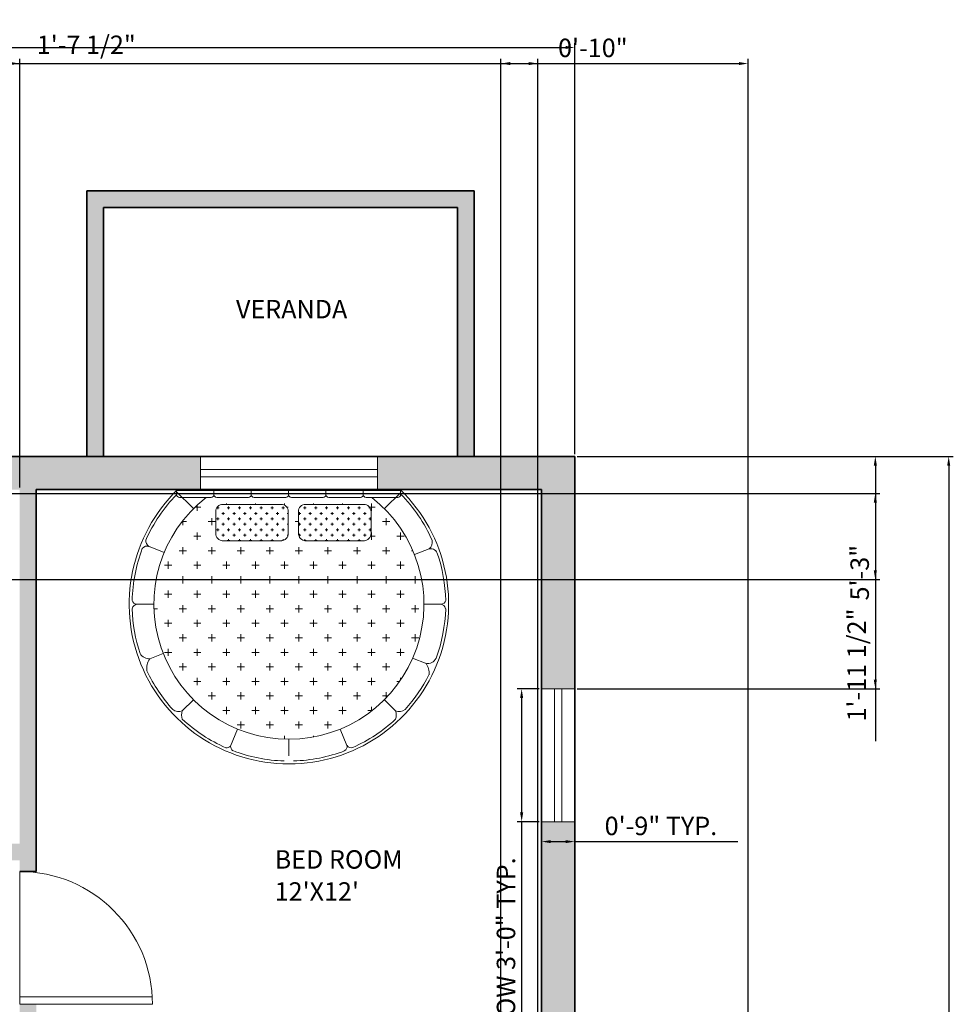
# Model space of a CAD drawing. Units: inches. Extents: x 2923 to 3500, y 1684 to 2381.
# Tile 12 of 12: x 3247 to 3500, y 2114 to 2381. Entities that reach past the tile are written whole.
import ezdxf

# ---------------------------------------------------------------- set-up
doc = ezdxf.new("R2010")
doc.units = ezdxf.units.IN
for name, color, linetype, lineweight in [('A-ANNO-DIMS', 2, 'Continuous', 18), ('A-AREA-IDEN', 7, 'Continuous', 18), ('A-DOOR', 3, 'Continuous', 18), ('A-FURN-PATT', 8, 'Continuous', 13), ('A-GLAZ', 4, 'Continuous', 18), ('A-WALL', 7, 'Continuous', 35), ('A-WALL-PATT', 9, 'Continuous', 13), ('Furniture', 7, 'Continuous', 15)]:
    doc.layers.add(name, color=color, linetype=linetype, lineweight=lineweight)
doc.styles.get("Standard").update_dxf_attribs({"font": 'txt', "height": 5})
doc.dimstyles.new('ISO-25', dxfattribs={"dimtxt": 5, "dimasz": 2.5, "dimexe": 1.25, "dimexo": 0.625, "dimtad": 1, "dimlunit": 3, "dimtxsty": 'Standard', "dimcen": 2.5, "dimadec": 0, "dimazin": 0, "dimtfac": 1, "dimtmove": 0, "dimatfit": 3, "dimfxl": 1, "dimarcsym": 0})

# ---------------------------------------------------------------- blocks, each defined once
blk = doc.blocks.new('*D2')
at = {"layer": 'A-ANNO-DIMS', "color": 0, "lineweight": -2, "transparency": 16777216}
for p, q in [((2969.23, 2263.03), (2969.23, 2374.52)), ((2971.73, 2373.27), (3394.73, 2373.27)), ((3397.23, 2263.03), (3397.23, 2374.52))]:
    blk.add_line(p, q, dxfattribs=at)
at = {"layer": 'A-ANNO-DIMS', "color": 0, "transparency": 16777216}
for points in [[(2971.73, 2373.69), (2971.73, 2372.86), (2969.23, 2373.27)], [(3394.73, 2373.69), (3394.73, 2372.86), (3397.23, 2373.27)]]:
    blk.add_solid(points, dxfattribs=at)
at = {"layer": 'Defpoints', "color": 0, "transparency": 16777216}
for p in [(3397.23, 2373.27), (2969.23, 2262.41), (3397.23, 2262.41)]:
    blk.add_point(p, dxfattribs=at)
at = {"layer": 'A-ANNO-DIMS', "color": 0, "transparency": 16777216, "insert": (3183.23, 2376.87), "char_height": 5, "attachment_point": 5}
blk.add_mtext('35\'-8"', dxfattribs=at)
blk = doc.blocks.new('*D3')
at = {"layer": 'A-ANNO-DIMS', "color": 0, "lineweight": -2, "transparency": 16777216}
for p, q in [((3397.85, 2262.41), (3499.87, 2262.41)), ((3498.62, 2259.91), (3498.62, 1819.91)), ((3397.85, 1817.41), (3499.87, 1817.41))]:
    blk.add_line(p, q, dxfattribs=at)
at = {"layer": 'A-ANNO-DIMS', "color": 0, "transparency": 16777216}
for points in [[(3498.2, 2259.91), (3499.04, 2259.91), (3498.62, 2262.41)], [(3498.2, 1819.91), (3499.04, 1819.91), (3498.62, 1817.41)]]:
    blk.add_solid(points, dxfattribs=at)
at = {"layer": 'Defpoints', "color": 0, "transparency": 16777216}
for p in [(3397.23, 2262.41), (3397.23, 1817.41), (3498.62, 1817.41)]:
    blk.add_point(p, dxfattribs=at)
at = {"layer": 'A-ANNO-DIMS', "color": 0, "transparency": 16777216, "insert": (3495.02, 2039.91), "char_height": 5, "attachment_point": 5, "rotation": 90}
blk.add_mtext('37\'-1"', dxfattribs=at)
blk = doc.blocks.new('DOOR-SINGLE-36IN')
for p, q in [((36, 36), (0, 36)), ((34, 0.06), (34, 36)), ((36, 0), (36, 36))]:
    blk.add_line(p, q)
blk.add_arc((36, 36), 36, 180, 270)
blk = doc.blocks.new('WINDOW-36IN')
for p, q in [((36, 9), (0, 9)), ((0, 9), (0, 0)), ((36, 0), (36, 9)), ((36, 5.5), (0, 5.5)), ((36, 3.5), (0, 3.5)), ((0, 0), (36, 0))]:
    blk.add_line(p, q)
blk = doc.blocks.new('VERANDA-PARAPET')
for p, q in [((0, 72), (0, 0)), ((4.5, 72), (4.5, 4.5)), ((100.5, 72), (100.5, 4.5)), ((105, 72), (105, 0)), ((100.5, 4.5), (4.5, 4.5)), ((105, 0), (0, 0))]:
    blk.add_line(p, q)
blk = doc.blocks.new('BED-ROUND-FRAME')
for p, q in [((31.04, 79.92), (31.04, 84.58)), ((31.04, 79.92), (31.04, 84.58)), ((17.61, 77.37), (16.05, 81.29)), ((45.66, 76.84), (47.11, 80.49)), ((0, 13.11), (0, 73.51)), ((5.15, 69.2), (0.74, 73.61)), ((5.15, 69.2), (0.74, 73.61)), ((56.93, 69.2), (59.95, 72.21)), ((56.93, 69.2), (59.95, 72.21)), ((59.95, 72.21), (56.93, 69.2)), ((13.83, 63.84), (13.83, 47.62)), ((64.9, 57.24), (69.31, 59.05)), ((69.31, 59.05), (69.4, 59.09)), ((67.65, 43.31), (72.18, 43.31)), ((13.83, 41.4), (13.83, 25.18)), ((13.83, 39.13), (13.84, 39.12)), ((64.9, 29.37), (69.53, 27.47)), ((0.42, 12.68), (5.15, 17.42)), ((0.42, 12.68), (5.15, 17.42)), ((59.95, 14.4), (56.93, 17.42)), ((17.07, 9.46), (15.35, 5.25)), ((44.42, 9.23), (45.86, 5.58)), ((31.04, 1.98), (31.04, 6.69)), ((31.04, 2.04), (31.04, 6.69))]:
    blk.add_line(p, q)
for points in [[(4, 47.85), (4, 63.6, -0.414214), (5.97, 65.57), (11.88, 65.57, -0.414214), (13.84, 63.6), (13.84, 47.85, -0.414214), (11.88, 45.89), (5.97, 45.89, -0.414214)], [(4, 25.41), (4, 41.16, -0.414214), (5.97, 43.13), (11.88, 43.13, -0.414214), (13.84, 41.16), (13.84, 25.41, -0.414214), (11.88, 23.45), (5.97, 23.45, -0.414214)]]:
    blk.add_lwpolyline(points, format="xyb", close=True)
for centre, radius, start, end in [((31.04, 43.31), 43.31, 224.213, 135.787), ((31.04, 43.31), 42.52, 91.3819, 109.0292), ((29.76, 84.56), 1.29, 359.0498, 78.348), ((32.5, 84.36), 1.46, 98.688, 183.9778), ((31.04, 43.31), 42.52, 69.8397, 88.3303), ((17.88, 81.76), 1.88, 111.9527, 202.5488), ((44.67, 80.98), 2.46, 345.7709, 65.4979), ((31.04, 43.31), 42.52, 114.0695, 134.5949), ((14.23, 79.9), 2.29, 37.3562, 103.3498), ((49.64, 77.03), 4.29, 82.908, 126.1659), ((31.04, 43.31), 42.52, 47.802, 63.2705), ((31.04, 43.31), 36.61, 217.8198, 142.1802), ((57.53, 73.21), 2.61, 337.5919, 37.6583), ((61.1, 69.09), 3.33, 70.4217, 110.1689), ((31.04, 43.31), 42.52, 24.0703, 42.854), ((69.6, 57.73), 1.36, 26.1665, 102.6069), ((68.6, 60.18), 1.35, 304.4266, 20.4145), ((31.04, 43.31), 42.52, 1.7281, 20.7271), ((31.04, 43.31), 42.52, 339.0428, 358.2719), ((69.4, 29.21), 1.75, 274.2316, 320.4352), ((68.35, 26.36), 1.62, 353.6066, 43.1756), ((31.04, 43.31), 42.52, 317.146, 336.245), ((57.53, 13.4), 2.61, 322.3417, 22.4081), ((61.1, 17.52), 3.33, 249.8311, 289.5783), ((31.04, 43.31), 42.52, 225.7269, 245.8957), ((31.04, 43.31), 42.52, 295.113, 312.198), ((16.89, 4.85), 1.59, 153.9459, 235.5493), ((42.79, 5.51), 3.04, 302.4304, 3.4261), ((48.39, 9.04), 4.29, 233.8341, 279.2916), ((13.85, 6.32), 1.83, 264.4179, 326.0029), ((31.04, 43.31), 42.52, 249.2703, 268.6181), ((31.04, 43.31), 42.52, 271.6697, 288.3347), ((29.76, 2.06), 1.29, 281.652, 0.9502), ((32.5, 2.25), 1.46, 176.0222, 261.312)]:
    blk.add_arc(centre, radius, start, end)
blk = doc.blocks.new('*D19')
at = {"layer": 'A-ANNO-DIMS', "color": 0, "lineweight": -2, "transparency": 16777216}
for p, q in [((3387.6, 2199.41), (3381.58, 2199.41)), ((3382.83, 2196.91), (3382.83, 2165.91)), ((3387.6, 2163.41), (3381.58, 2163.41)), ((3382.83, 2163.41), (3382.83, 2085.85))]:
    blk.add_line(p, q, dxfattribs=at)
at = {"layer": 'A-ANNO-DIMS', "color": 0, "transparency": 16777216}
for points in [[(3382.41, 2196.91), (3383.25, 2196.91), (3382.83, 2199.41)], [(3382.41, 2165.91), (3383.25, 2165.91), (3382.83, 2163.41)]]:
    blk.add_solid(points, dxfattribs=at)
at = {"layer": 'Defpoints', "color": 0, "transparency": 16777216}
for p in [(3388.23, 2199.41), (3382.83, 2163.41), (3388.23, 2163.41)]:
    blk.add_point(p, dxfattribs=at)
at = {"layer": 'A-ANNO-DIMS', "color": 0, "transparency": 16777216, "insert": (3379.23, 2123.38), "char_height": 5, "attachment_point": 5, "rotation": 90}
blk.add_mtext('WINDOW 3\'-0" TYP.', dxfattribs=at)
blk = doc.blocks.new('*D20')
at = {"layer": 'A-ANNO-DIMS', "color": 0, "lineweight": -2, "transparency": 16777216}
for p, q in [((3388.23, 2162.78), (3388.23, 2156.76)), ((3397.23, 2162.78), (3397.23, 2156.76)), ((3390.73, 2158.01), (3394.73, 2158.01)), ((3397.23, 2158.01), (3441.46, 2158.01))]:
    blk.add_line(p, q, dxfattribs=at)
at = {"layer": 'A-ANNO-DIMS', "color": 0, "transparency": 16777216}
for points in [[(3390.73, 2158.42), (3390.73, 2157.59), (3388.23, 2158.01)], [(3394.73, 2158.42), (3394.73, 2157.59), (3397.23, 2158.01)]]:
    blk.add_solid(points, dxfattribs=at)
at = {"layer": 'Defpoints', "color": 0, "transparency": 16777216}
for p in [(3388.23, 2163.41), (3397.23, 2163.41), (3397.23, 2158.01)]:
    blk.add_point(p, dxfattribs=at)
at = {"layer": 'A-ANNO-DIMS', "color": 0, "transparency": 16777216, "insert": (3420.59, 2161.61), "char_height": 5, "attachment_point": 5}
blk.add_mtext('0\'-9" TYP.', dxfattribs=at)
blk = doc.blocks.new('*D49')
at = {"layer": 'A-ANNO-DIMS', "color": 0, "lineweight": -2, "transparency": 16777216}
for p, q in [((2969.23, 2263.03), (2969.23, 2370.16)), ((3444.23, 2110.03), (3444.23, 2370.16)), ((2971.73, 2368.91), (3441.73, 2368.91))]:
    blk.add_line(p, q, dxfattribs=at)
at = {"layer": 'A-ANNO-DIMS', "color": 0, "transparency": 16777216}
for points in [[(2971.73, 2369.32), (2971.73, 2368.49), (2969.23, 2368.91)], [(3441.73, 2369.32), (3441.73, 2368.49), (3444.23, 2368.91)]]:
    blk.add_solid(points, dxfattribs=at)
at = {"layer": 'Defpoints', "color": 0, "transparency": 16777216}
for p in [(3444.23, 2368.91), (2969.23, 2262.41), (3444.23, 2109.41)]:
    blk.add_point(p, dxfattribs=at)
at = {"layer": 'A-ANNO-DIMS', "color": 0, "transparency": 16777216, "insert": (3206.73, 2372.51), "char_height": 5, "attachment_point": 5}
blk.add_mtext('39\'-7"', dxfattribs=at)
blk = doc.blocks.new('*D53')
at = {"layer": 'A-ANNO-DIMS', "color": 0, "lineweight": -2, "transparency": 16777216}
for p, q in [((3153.3, 2254.03), (3153.3, 2370.16)), ((3246.73, 2254.03), (3246.73, 2370.16)), ((3155.8, 2368.91), (3244.23, 2368.91))]:
    blk.add_line(p, q, dxfattribs=at)
at = {"layer": 'A-ANNO-DIMS', "color": 0, "transparency": 16777216}
for points in [[(3155.8, 2369.32), (3155.8, 2368.49), (3153.3, 2368.91)], [(3244.23, 2369.32), (3244.23, 2368.49), (3246.73, 2368.91)]]:
    blk.add_solid(points, dxfattribs=at)
at = {"layer": 'Defpoints', "color": 0, "transparency": 16777216}
for p in [(3246.73, 2368.91), (3153.3, 2253.41), (3246.73, 2253.41)]:
    blk.add_point(p, dxfattribs=at)
at = {"layer": 'A-ANNO-DIMS', "color": 0, "transparency": 16777216, "insert": (3200.02, 2373.34), "char_height": 5, "attachment_point": 5}
blk.add_mtext('7\'-9 1/2"', dxfattribs=at)
blk = doc.blocks.new('*D56')
at = {"layer": 'A-ANNO-DIMS', "color": 0, "lineweight": -2, "transparency": 16777216}
for p, q in [((3223.64, 2253.03), (3223.64, 2370.16)), ((3243.09, 2253.03), (3243.09, 2370.16)), ((3226.14, 2368.91), (3240.59, 2368.91)), ((3243.09, 2368.91), (3283.99, 2368.91))]:
    blk.add_line(p, q, dxfattribs=at)
at = {"layer": 'A-ANNO-DIMS', "color": 0, "transparency": 16777216}
for points in [[(3226.14, 2369.32), (3226.14, 2368.49), (3223.64, 2368.91)], [(3240.59, 2369.32), (3240.59, 2368.49), (3243.09, 2368.91)]]:
    blk.add_solid(points, dxfattribs=at)
at = {"layer": 'Defpoints', "color": 0, "transparency": 16777216}
for p in [(3243.09, 2368.91), (3223.64, 2252.4), (3243.09, 2252.4)]:
    blk.add_point(p, dxfattribs=at)
at = {"layer": 'A-ANNO-DIMS', "color": 0, "transparency": 16777216, "insert": (3264.79, 2373.34), "char_height": 5, "attachment_point": 5}
blk.add_mtext('1\'-7 1/2"', dxfattribs=at)
blk = doc.blocks.new('*D57')
at = {"layer": 'A-ANNO-DIMS', "color": 0, "lineweight": -2, "transparency": 16777216}
for p, q in [((3243.72, 2252.4), (3479.98, 2252.4)), ((3478.73, 2249.9), (3478.73, 2231.51)), ((3243.72, 2229.01), (3479.98, 2229.01)), ((3478.73, 2229.01), (3478.73, 2185.26))]:
    blk.add_line(p, q, dxfattribs=at)
at = {"layer": 'A-ANNO-DIMS', "color": 0, "transparency": 16777216}
for points in [[(3478.31, 2249.9), (3479.15, 2249.9), (3478.73, 2252.4)], [(3478.31, 2231.51), (3479.15, 2231.51), (3478.73, 2229.01)]]:
    blk.add_solid(points, dxfattribs=at)
at = {"layer": 'Defpoints', "color": 0, "transparency": 16777216}
for p in [(3243.09, 2252.4), (3243.09, 2229.01), (3478.73, 2229.01)]:
    blk.add_point(p, dxfattribs=at)
at = {"layer": 'A-ANNO-DIMS', "color": 0, "transparency": 16777216, "insert": (3474.3, 2205.88), "char_height": 5, "attachment_point": 5, "rotation": 90}
blk.add_mtext('1\'-11 1/2"', dxfattribs=at)
blk = doc.blocks.new('*D70')
at = {"layer": 'A-ANNO-DIMS', "color": 0, "lineweight": -2, "transparency": 16777216}
for p, q in [((3397.85, 2262.41), (3479.98, 2262.41)), ((3478.73, 2259.91), (3478.73, 2201.91)), ((3397.85, 2199.41), (3479.98, 2199.41))]:
    blk.add_line(p, q, dxfattribs=at)
at = {"layer": 'A-ANNO-DIMS', "color": 0, "transparency": 16777216}
for points in [[(3478.31, 2259.91), (3479.15, 2259.91), (3478.73, 2262.41)], [(3478.31, 2201.91), (3479.15, 2201.91), (3478.73, 2199.41)]]:
    blk.add_solid(points, dxfattribs=at)
at = {"layer": 'Defpoints', "color": 0, "transparency": 16777216}
for p in [(3397.23, 2262.41), (3397.23, 2199.41), (3478.73, 2199.41)]:
    blk.add_point(p, dxfattribs=at)
at = {"layer": 'A-ANNO-DIMS', "color": 0, "transparency": 16777216, "insert": (3475.13, 2230.91), "char_height": 5, "attachment_point": 5, "rotation": 90}
blk.add_mtext('5\'-3"', dxfattribs=at)
blk = doc.blocks.new('*D71')
at = {"layer": 'A-ANNO-DIMS', "color": 0, "lineweight": -2, "transparency": 16777216}
for p, q in [((3377.23, 2105.53), (3377.23, 2370.16)), ((3387.23, 2105.53), (3387.23, 2370.16)), ((3379.73, 2368.91), (3384.73, 2368.91)), ((3387.23, 2368.91), (3414.55, 2368.91))]:
    blk.add_line(p, q, dxfattribs=at)
at = {"layer": 'A-ANNO-DIMS', "color": 0, "transparency": 16777216}
for points in [[(3379.73, 2369.32), (3379.73, 2368.49), (3377.23, 2368.91)], [(3384.73, 2369.32), (3384.73, 2368.49), (3387.23, 2368.91)]]:
    blk.add_solid(points, dxfattribs=at)
at = {"layer": 'Defpoints', "color": 0, "transparency": 16777216}
for p in [(3387.23, 2368.91), (3377.23, 2104.91), (3387.23, 2104.91)]:
    blk.add_point(p, dxfattribs=at)
at = {"layer": 'A-ANNO-DIMS', "color": 0, "transparency": 16777216, "insert": (3402.14, 2372.51), "char_height": 5, "attachment_point": 5}
blk.add_mtext('0\'-10"', dxfattribs=at)

msp = doc.modelspace()

# ---------------------------------------------------------------- hatches: boundary and pattern name
at = {"layer": 'A-FURN-PATT'}
h = msp.add_hatch(dxfattribs=at)
h.set_pattern_fill('CROSS', color=256, scale=15.748, angle=90, style=0)
h.set_pattern_definition([(270, (1810.6367, 3985.8724), (-3.937, -3.937), [1.9685, -5.9055]), (180, (1811.621, 3984.888), (-3.937, 3.937), [1.9685, -5.9055])])
h.paths.add_polyline_path([(3342.181, 2251.289), (3340.635, 2251.289, -0.4142136), (3339.887, 2252.037, -0.4142136), (3339.139, 2251.289), (3330.515, 2251.289, -0.4142136), (3329.767, 2252.037, -0.4142136), (3329.019, 2251.289), (3320.394, 2251.289, -0.4142136), (3319.646, 2252.037, -0.4142136), (3318.898, 2251.289), (3310.274, 2251.289, -0.4142136), (3309.526, 2252.037, -0.4142136), (3308.778, 2251.289), (3300.153, 2251.289, -0.4142136), (3299.405, 2252.037, -0.4142136), (3298.657, 2251.289), (3297.279, 2251.289, 2.9191153)])
h.paths.add_polyline_path([(3301.836, 2239.562, -0.4142136), (3299.868, 2241.531), (3299.868, 2247.436, -0.4142136), (3301.836, 2249.405), (3317.584, 2249.405, -0.4142136), (3319.553, 2247.436), (3319.553, 2241.531, -0.4142136), (3317.584, 2239.562)], flags=16)
h.paths.add_polyline_path([(3322.309, 2241.531), (3322.309, 2247.436, -0.4142136), (3324.277, 2249.405), (3340.025, 2249.405, -0.4142136), (3341.994, 2247.436), (3341.994, 2241.531, -0.4142136), (3340.025, 2239.562), (3324.277, 2239.562, -0.4142136)], flags=16)
h = msp.add_hatch(dxfattribs=at)
h.set_pattern_fill('CROSS', color=256, scale=5.9055, angle=360, style=0)
h.set_pattern_definition([(1e-14, (2643.0597, 1508.7883), (1.476375, 1.476375), [0.7381875, -2.2145625]), (90, (2643.4288, 1508.4192), (-1.476375, 1.476375), [0.7381875, -2.2145625])])
h.paths.add_polyline_path([(3301.836, 2249.405, 0.4142136), (3299.868, 2247.436), (3299.868, 2241.531, 0.4142136), (3301.836, 2239.562), (3317.584, 2239.562, 0.4142136), (3319.553, 2241.531), (3319.553, 2247.436, 0.4142136), (3317.584, 2249.405)])
h.paths.add_polyline_path([(3340.025, 2239.562, 0.4142136), (3341.994, 2241.531), (3341.994, 2247.436, 0.4142136), (3340.025, 2249.405), (3324.277, 2249.405, 0.4142136), (3322.309, 2247.436), (3322.309, 2241.531, 0.4142136), (3324.277, 2239.562)])
at = {"layer": 'A-WALL-PATT'}
h = msp.add_hatch(color=256, dxfattribs=at)
h.dxf.hatch_style = 1
h.paths.add_polyline_path([(3014.23, 2262.406), (2969.23, 2262.406), (2969.23, 2201.5), (2978.23, 2201.5), (2978.23, 2213.699), (2978.23, 2253.406), (3014.23, 2253.406)])
h.paths.add_polyline_path([(3119.23, 2262.406), (3074.23, 2262.406), (3074.23, 2253.406), (3110.23, 2253.406), (3110.23, 2109.406), (3105.73, 2109.406), (3105.73, 2104.906), (3114.73, 2104.906), (3114.73, 2152.906), (3119.23, 2152.906), (3119.23, 2157.406), (3114.73, 2157.406), (3114.73, 2253.406), (3119.23, 2253.406)])
h.paths.add_polyline_path([(3179.98, 2262.406), (3149.23, 2262.406), (3149.23, 2253.406), (3179.98, 2253.406)], flags=0)
h.paths.add_polyline_path([(3295.73, 2262.406), (3215.98, 2262.406), (3215.98, 2253.406), (3246.73, 2253.406), (3246.73, 2157.406), (3149.23, 2157.406), (3149.23, 2152.906), (3246.73, 2152.906), (3246.73, 2149.906), (3251.23, 2149.906), (3251.23, 2253.406), (3295.73, 2253.406)])
h.paths.add_polyline_path([(3397.23, 2262.406), (3343.73, 2262.406), (3343.73, 2253.406), (3349.929, 2253.406), (3388.23, 2253.406), (3388.23, 2199.406), (3397.23, 2199.406)])
h.paths.add_polyline_path([(3369.935, 2334.406), (3264.935, 2334.406), (3264.935, 2262.406), (3269.435, 2262.406), (3269.435, 2329.906), (3365.435, 2329.906), (3365.435, 2262.406), (3369.935, 2262.406)])
h.paths.add_polyline_path([(3096.73, 2334.406), (2991.73, 2334.406), (2991.73, 2262.406), (2996.23, 2262.406), (2996.23, 2329.906), (3092.23, 2329.906), (3092.23, 2262.406), (3096.73, 2262.406)])
h.paths.add_polyline_path([(3397.23, 2163.406), (3388.23, 2163.406), (3388.23, 2109.406), (3251.23, 2109.406), (3251.23, 2113.906), (3246.73, 2113.906), (3246.73, 2092.906), (3251.23, 2092.906), (3251.23, 2104.906), (3435.23, 2104.906), (3435.23, 2080.906), (3444.23, 2080.906), (3444.23, 2109.406), (3397.23, 2109.406)])
h.paths.add_polyline_path([(3444.23, 2044.906), (3435.23, 2044.906), (3435.23, 2020.906), (3251.23, 2020.906), (3251.23, 2032.906), (3246.73, 2032.906), (3246.73, 2016.406), (3251.23, 2016.406), (3287.73, 2016.406), (3287.73, 1968.406), (3287.23, 1968.406), (3287.23, 1963.906), (3296.73, 1963.906), (3296.73, 1968.406), (3292.23, 1968.406), (3292.23, 2016.406), (3388.23, 2016.406), (3388.23, 2004.398), (3397.23, 2004.398), (3397.23, 2016.406), (3444.23, 2016.406)])
h.paths.add_polyline_path([(3397.23, 1980.398), (3388.23, 1980.398), (3388.23, 1979.998), (3388.23, 1969.828), (3388.23, 1968.406), (3326.73, 1968.406), (3326.73, 1963.906), (3388.23, 1963.906), (3388.23, 1913.156), (3397.23, 1913.156)])
h.paths.add_polyline_path([(3251.23, 1968.406), (3150.73, 1968.406), (3150.73, 1963.906), (3246.73, 1963.906), (3246.73, 1826.406), (3230.98, 1826.406), (3230.98, 1817.406), (3251.23, 1817.406), (3251.23, 1963.906)])
h.paths.add_polyline_path([(3114.73, 1968.406), (3105.73, 1968.406), (3105.73, 1963.906), (3110.23, 1963.906), (3110.23, 1817.406), (3119.23, 1817.406), (3119.23, 1826.406), (3114.73, 1826.406)])
h.paths.add_polyline_path([(3069.73, 1968.406), (3066.73, 1968.406), (3066.73, 1972.906), (3062.23, 1972.906), (3062.23, 1968.406), (2978.23, 1968.406), (2978.23, 1989.406), (2969.23, 1989.406), (2969.23, 1912.505), (2978.23, 1912.505), (2978.23, 1925.355), (2978.23, 1963.906), (3069.73, 1963.906)])
h.paths.add_polyline_path([(3066.73, 2104.906), (3069.73, 2104.906), (3069.73, 2109.406), (3057.73, 2109.406), (3057.73, 2104.906), (3062.23, 2104.906), (3062.23, 2038.906), (2978.23, 2038.906), (2978.23, 2059.906), (2969.23, 2059.906), (2969.23, 2013.406), (2978.23, 2013.406), (2978.23, 2034.406), (3062.23, 2034.406), (3062.23, 2002.906), (3066.73, 2002.906)])
h.paths.add_polyline_path([(3027.73, 2109.406), (2978.23, 2109.406), (2978.23, 2165.5), (2969.23, 2165.5), (2969.23, 2083.906), (2978.23, 2083.906), (2978.23, 2104.906), (3027.73, 2104.906)])
h.paths.add_polyline_path([(2978.23, 1876.505), (2969.23, 1876.505), (2969.23, 1817.406), (3014.23, 1817.406), (3014.23, 1826.406), (2978.23, 1826.406)])
h.paths.add_polyline_path([(2996.23, 1817.406), (2991.73, 1817.406), (2991.73, 1745.406), (3096.73, 1745.406), (3096.73, 1817.406), (3092.23, 1817.406), (3092.23, 1749.906), (2996.23, 1749.906)])
h.paths.add_polyline_path([(3289.73, 1826.406), (3251.23, 1826.406), (3251.23, 1817.406), (3289.73, 1817.406)])
h.paths.add_polyline_path([(3397.23, 1877.156), (3388.23, 1877.156), (3388.23, 1864.957), (3388.23, 1826.406), (3349.73, 1826.406), (3349.73, 1817.406), (3397.23, 1817.406)])
h.paths.add_polyline_path([(3374.267, 1817.406), (3369.767, 1817.406), (3369.767, 1749.906), (3273.767, 1749.906), (3273.767, 1817.406), (3269.267, 1817.406), (3269.267, 1745.406), (3374.267, 1745.406)])

# ---------------------------------------------------------------- linework, layer by layer
at = {"layer": 'A-GLAZ'}
for p, q in [((3343.73, 2262.406), (3295.73, 2262.406)), ((3295.73, 2262.406), (3295.73, 2253.406)), ((3343.73, 2253.406), (3343.73, 2262.406)), ((3343.73, 2258.906), (3295.73, 2258.906)), ((3343.73, 2256.906), (3295.73, 2256.906)), ((3295.73, 2253.406), (3343.73, 2253.406))]:
    msp.add_line(p, q, dxfattribs=at)
at = {"layer": 'A-WALL'}
for p, q in [((3149.23, 2262.406), (3397.23, 2262.406)), ((3397.23, 2262.406), (3397.23, 2109.406)), ((3251.23, 2253.406), (3388.23, 2253.406)), ((3251.23, 2149.906), (3251.23, 2253.406)), ((3388.23, 2253.406), (3388.23, 2109.406)), ((3251.23, 2149.906), (3246.73, 2149.906))]:
    msp.add_line(p, q, dxfattribs=at)
at = {"layer": 'Furniture'}
for points in [[(3290.033, 2251.289), (3298.657, 2251.289, 0.4142136), (3299.405, 2252.037), (3299.405, 2253.178), (3289.285, 2253.178), (3289.285, 2252.037, 0.4142136)], [(3300.153, 2251.289), (3308.778, 2251.289, 0.4142136), (3309.526, 2252.037), (3309.526, 2253.178), (3299.405, 2253.178), (3299.405, 2252.037, 0.4142136)], [(3310.274, 2251.289), (3318.898, 2251.289, 0.4142136), (3319.646, 2252.037), (3319.646, 2253.178), (3309.526, 2253.178), (3309.526, 2252.037, 0.4142136)], [(3320.394, 2251.289), (3329.019, 2251.289, 0.4142136), (3329.767, 2252.037), (3329.767, 2253.178), (3319.646, 2253.178), (3319.646, 2252.037, 0.4142136)], [(3330.515, 2251.289), (3339.139, 2251.289, 0.4142136), (3339.887, 2252.037), (3339.887, 2253.178), (3329.767, 2253.178), (3329.767, 2252.037, 0.4142136)], [(3340.635, 2251.289), (3349.26, 2251.289, 0.4142136), (3350.008, 2252.037), (3350.008, 2253.178), (3339.887, 2253.178), (3339.887, 2252.037, 0.4142136)]]:
    msp.add_lwpolyline(points, format="xyb", close=True, dxfattribs=at)

# ---------------------------------------------------------------- block references
at = {"layer": 'A-DOOR', "extrusion": (0, 0, -1), "zscale": -1, "rotation": 269.9999999999997}
msp.add_blockref('DOOR-SINGLE-36IN', (-3282.73, 2149.906), dxfattribs=at)
at = {"layer": 'A-GLAZ', "rotation": 269.9999999999986}
msp.add_blockref('WINDOW-36IN', (3388.23, 2199.406), dxfattribs=at)
at = {"layer": 'A-WALL', "rotation": 180}
msp.add_blockref('VERANDA-PARAPET', (3369.934, 2334.406), dxfattribs=at)
at = {"layer": 'Furniture', "rotation": 269.9998213702181}
msp.add_blockref('BED-ROUND-FRAME', (3276.423, 2253.406), dxfattribs=at)

# ---------------------------------------------------------------- texts
at = {"layer": 'A-AREA-IDEN'}
for s, p in [('VERANDA', (3305.375, 2299.833)), ('BED ROOM', (3315.866, 2150.676)), ("12'X12'", (3315.866, 2141.991))]:
    msp.add_text(s, height=5, dxfattribs=at).set_placement(p)

# ---------------------------------------------------------------- dimensions: what is measured, and where the dimension line sits
at = {"layer": 'A-ANNO-DIMS'}
for base, p1, p2, override, picture, middle in [((3246.73, 2368.906), (3153.303, 2253.406), (3246.73, 2253.406), {"dimdec": 1, "dimlfac": 1, "dimrnd": 0, "dimzin": 1, "dimdsep": 46, "dimlunit": 4, "dimfrac": 2}, '*D53', (3200.016, 2373.341)), ((3243.095, 2368.906), (3223.64, 2252.401), (3243.095, 2252.401), {"dimdec": 1, "dimlfac": 1, "dimrnd": 0, "dimzin": 1, "dimdsep": 46, "dimlunit": 4, "dimfrac": 2}, '*D56', (3264.791, 2373.341)), ((3397.23, 2373.272), (2969.23, 2262.406), (3397.23, 2262.406), {"dimclrd": 0, "dimclre": 0, "dimclrt": 0}, '*D2', (3183.23, 2376.874)), ((3444.23, 2368.906), (2969.23, 2262.406), (3444.23, 2109.406), {"dimdec": 1, "dimlfac": 1, "dimrnd": 0, "dimzin": 1, "dimdsep": 46, "dimlunit": 4, "dimfrac": 2}, '*D49', (3206.73, 2372.507)), ((3387.23, 2368.906), (3377.23, 2104.906), (3387.23, 2104.906), {"dimdec": 1, "dimlfac": 1, "dimrnd": 0, "dimzin": 1, "dimdsep": 46, "dimlunit": 4, "dimfrac": 2}, '*D71', (3402.141, 2372.507))]:
    dim = msp.add_linear_dim(base=base, p1=p1, p2=p2, dimstyle='ISO-25', override=override, dxfattribs=at)
    dim.commit()
    dim.dimension.update_dxf_attribs({"geometry": picture, "text_midpoint": middle})
for base, p1, p2, override, picture, middle in [((3498.62, 1817.406), (3397.23, 2262.406), (3397.23, 1817.406), {"dimclrd": 0, "dimclre": 0, "dimclrt": 0}, '*D3', (3495.019, 2039.906)), ((3478.73, 2199.406), (3397.23, 2262.406), (3397.23, 2199.406), {"dimdec": 1, "dimlfac": 1, "dimrnd": 0, "dimzin": 1, "dimdsep": 46, "dimlunit": 4, "dimfrac": 2}, '*D70', (3475.129, 2230.906)), ((3478.73, 2229.01), (3243.095, 2252.401), (3243.095, 2229.01), {"dimdec": 1, "dimlfac": 1, "dimrnd": 0, "dimzin": 1, "dimdsep": 46, "dimlunit": 4, "dimfrac": 2}, '*D57', (3474.295, 2205.885))]:
    dim = msp.add_linear_dim(base=base, p1=p1, p2=p2, angle=90, dimstyle='ISO-25', override=override, dxfattribs=at)
    dim.commit()
    dim.dimension.update_dxf_attribs({"geometry": picture, "text_midpoint": middle})
dim = msp.add_linear_dim(base=(3382.83, 2163.406), p1=(3388.23, 2199.406), p2=(3388.23, 2163.406), angle=270, text='WINDOW <> TYP.', dimstyle='ISO-25', override={"dimdec": 1, "dimlfac": 1, "dimrnd": 0, "dimzin": 1, "dimdsep": 46, "dimlunit": 4, "dimfrac": 2}, dxfattribs=at)
dim.commit()
dim.dimension.update_dxf_attribs({"geometry": '*D19', "text_midpoint": (3379.229, 2123.376)})
dim = msp.add_linear_dim(base=(3397.23, 2158.006), p1=(3388.23, 2163.406), p2=(3397.23, 2163.406), text='<> TYP.', dimstyle='ISO-25', override={"dimdec": 1, "dimlfac": 1, "dimrnd": 0, "dimzin": 1, "dimdsep": 46, "dimlunit": 4, "dimfrac": 2}, dxfattribs=at)
dim.commit()
dim.dimension.update_dxf_attribs({"geometry": '*D20', "text_midpoint": (3420.593, 2161.607)})

doc.saveas('drawing.dxf')
